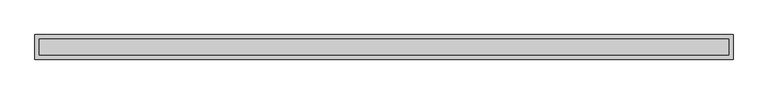
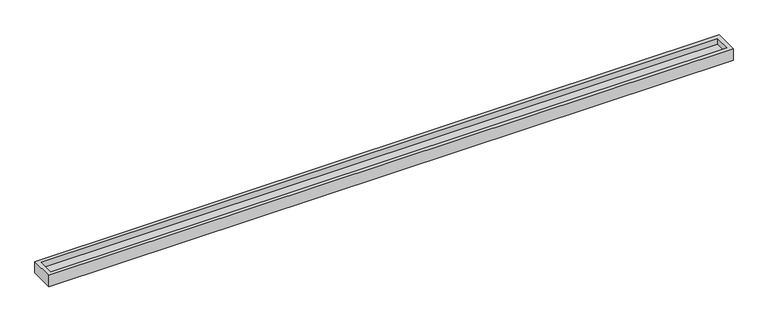
"""IFC4 building model written with IfcOpenShell, lengths in millimetres: proxy geometry."""

from ifc_helpers import new_model, si_unit, origin, place, context, project, spatial, faceted_brep, source, transform, mapped, element, save


def roads_ea5b5616(model_context):
    return source(origin(), model_context, "Body", "Brep", [
        faceted_brep([(-14667.2963079, -8349.8760916, -1676.4), (-31990.0963079, -8349.8760916, -1676.4), (-31990.0963079, -8960.3102169, -1676.4), (-14667.2963079, -8960.3102169, -1676.4), (-14768.8963079, -8451.4760916, -1676.4), (-14768.8963079, -8858.7102169, -1676.4), (-31888.4963079, -8858.7102169, -1676.4), (-31888.4963079, -8451.4760916, -1676.4), (-14667.2963079, -8349.8760916, -1981.2), (-14667.2963079, -8960.3102169, -1981.2), (-31990.0963079, -8960.3102169, -1981.2), (-31990.0963079, -8349.8760916, -1981.2), (-14768.8963079, -8451.4760916, -1828.8), (-31888.4963079, -8451.4760916, -1828.8), (-31888.4963079, -8858.7102169, -1828.8), (-14768.8963079, -8858.7102169, -1828.8)], [[[0, 1, 2, 3], [4, 5, 6, 7]], [[8, 9, 10, 11]], [[1, 0, 8, 11]], [[2, 1, 11, 10]], [[3, 2, 10, 9]], [[0, 3, 9, 8]], [[12, 13, 14, 15]], [[12, 15, 5, 4]], [[15, 14, 6, 5]], [[14, 13, 7, 6]], [[13, 12, 4, 7]]]),
    ])


if __name__ == "__main__":
    model = new_model("IFC4")
    model_context = context("Model", 3, world=origin())
    ifc_project = project(units=[si_unit("LENGTHUNIT", "METRE", prefix="MILLI")], contexts=[model_context])
    site = spatial("IfcSite", under=ifc_project)
    building = spatial("IfcBuilding", under=site)
    placement = place(None, origin())
    roads_shape = roads_ea5b5616(model_context)
    element("IfcBuildingElementProxy", 1, Name="Roads", at=placement, inside=building, context=model_context, shape_type="MappedRepresentation", body=[
        mapped(roads_shape, transform((0.0, 0.0, 0.0), x_axis=(1.0, 0.0, 0.0), y_axis=(0.0, 1.0, 0.0), z_axis=(0.0, 0.0, 1.0))),
    ])
    save(model, "model.ifc")
